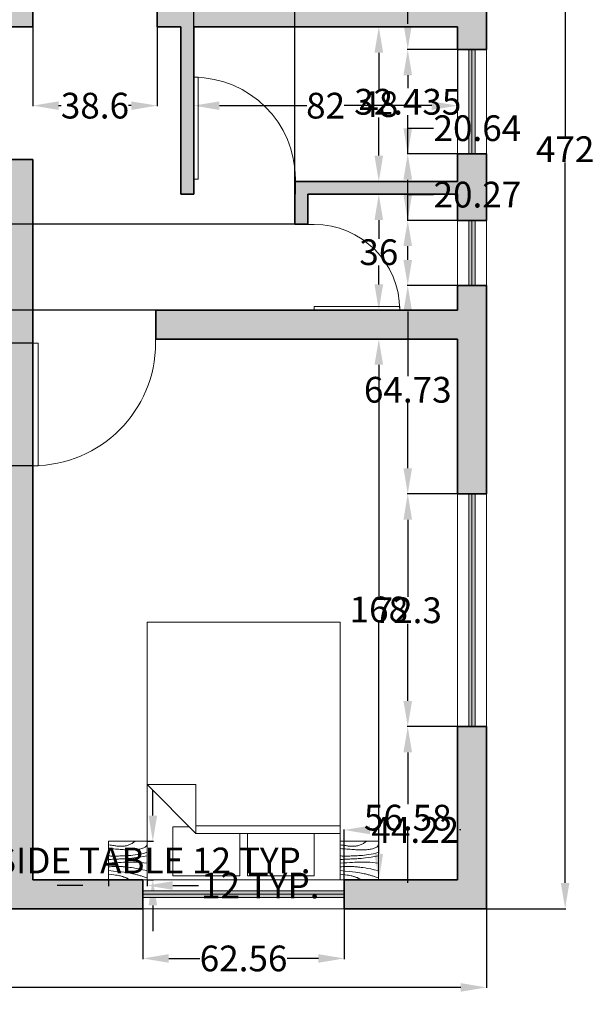
# Model space of a CAD drawing. Units: inches. Extents: x -52 to 678, y 23 to 685.
# Tile 10 of 11: x 431 to 609, y 23 to 329. Entities that reach past the tile are written whole.
import ezdxf

# ---------------------------------------------------------------- set-up
doc = ezdxf.new("R2010")
doc.units = ezdxf.units.IN
doc.header["$MEASUREMENT"] = 0
for name, color, linetype, lineweight in [('A-ANNO-DIMS', 2, 'Continuous', 18), ('A-DOOR', 3, 'Continuous', 18), ('A-FURN', 8, 'Continuous', 18), ('A-GLAZ', 4, 'Continuous', 18), ('A-WALL', 7, 'Continuous', 35)]:
    doc.layers.add(name, color=color, linetype=linetype, lineweight=lineweight)
doc.layers.add('A-GLAZ-PATT', color=18, linetype='Continuous', lineweight=13, true_color=0x000000)
doc.layers.add('A-WALL-PATT', color=18, linetype='Continuous', lineweight=13, true_color=0x000000)
doc.styles.get("Standard").update_dxf_attribs({"font": 'arial.ttf'})
doc.dimstyles.get("Standard").update_dxf_attribs({"dimtxt": 8, "dimasz": 8, "dimexe": 0.18, "dimexo": 0.0625, "dimgap": 0.09, "dimtad": 0, "dimtih": 1, "dimtoh": 1, "dimdec": 0, "dimzin": 0, "dimdsep": 46, "dimlunit": 3, "dimtxsty": 'Standard', "dimcen": 0.09, "dimadec": 0, "dimazin": 0, "dimtfac": 1, "dimtdec": 0, "dimtofl": 0, "dimtmove": 0, "dimatfit": 3, "dimfxl": 1, "dimtolj": 1, "dimtzin": 0, "dimarcsym": 0})

# ---------------------------------------------------------------- blocks, each defined once
blk = doc.blocks.new('Bed - Queen')
for p, q in [((0, -80.00003), (0, 0)), ((0, 0), (59.99999, 0)), ((59.99999, 0), (59.99999, -80.00003)), ((7.99999, -1.2), (28.79998, -1.2)), ((7.99999, -14.4), (7.99999, -1.2)), ((28.79998, -1.2), (28.79998, -14.4)), ((31.19999, -1.2), (51.99999, -1.2)), ((31.19999, -14.4), (31.19999, -1.2)), ((51.99999, -1.2), (51.99999, -16.4)), ((0, -14.4), (44.8, -14.4)), ((59.99999, -29.6), (44.8, -14.4)), ((44.8, -14.4), (44.8, -29.6)), ((44.8, -16.8), (0, -16.8)), ((51.99999, -16.4), (46.79936, -16.4)), ((44.8, -29.6), (59.99999, -29.6)), ((59.99999, -80.00003), (0, -80.00003))]:
    blk.add_line(p, q)
blk = doc.blocks.new('Table - Square Woodgrain 42 x 42 in.')
blk.add_line((0, -42), (42, -42))
for points in [[(0, -4), (1.704, -4.2172), (3.2358, -4.4188), (4.615, -4.604), (5.8615, -4.7721), (6.9951, -4.9224), (8.0357, -5.0541), (9.0031, -5.1667), (9.9171, -5.2594), (10.7951, -5.3316), (11.6445, -5.3836), (12.4702, -5.4157), (13.277, -5.4283), (14.0698, -5.4217), (14.8535, -5.3964), (15.6331, -5.3526), (16.4133, -5.2908), (17.1986, -5.2103), (17.9913, -5.1062), (18.793, -4.9727), (19.6056, -4.8038), (20.4307, -4.5937), (21.2701, -4.3365), (22.1256, -4.0262), (22.9989, -3.6571), (23.888, -3.2272), (24.7756, -2.7516), (25.6408, -2.2491), (26.4624, -1.7387), (27.2195, -1.2395), (27.891, -0.7703), (28.456, -0.3501), (28.8934, 0.002)], [(0, -42), (0, 0), (42, 0), (42, -42)], [(0, -8), (1.8203, -8.1001), (3.6741, -8.2149), (5.5411, -8.3408), (7.4011, -8.4741), (9.2339, -8.6112), (11.0193, -8.7484), (12.7371, -8.8821), (14.3671, -9.0086), (15.8954, -9.1246), (17.3337, -9.2278), (18.6997, -9.3159), (20.0116, -9.387), (21.2871, -9.4389), (22.5442, -9.4696), (23.8008, -9.477), (25.0749, -9.459), (26.3791, -9.4137), (27.7049, -9.3403), (29.0383, -9.2382), (30.3655, -9.1068), (31.6728, -8.9455), (32.9461, -8.7535), (34.1717, -8.5304), (35.3358, -8.2756), (36.4268, -7.9863), (37.443, -7.6521), (38.3849, -7.2603), (39.253, -6.7986), (40.048, -6.2542), (40.7705, -5.6147), (41.421, -4.8674), (42, -4)], [(42, -12), (39.1784, -12.8621), (36.4519, -13.5654), (33.8246, -14.1294), (31.3004, -14.5731), (28.8832, -14.9161), (26.577, -15.1775), (24.3858, -15.3768), (22.3136, -15.5332), (20.3622, -15.6632), (18.5254, -15.7718), (16.7947, -15.8612), (15.1618, -15.9338), (13.6183, -15.9916), (12.1558, -16.0369), (10.7659, -16.0718), (9.4403, -16.0987), (8.1703, -16.1191), (6.9461, -16.1325), (5.7577, -16.1377), (4.595, -16.1335), (3.4479, -16.1188), (2.3064, -16.0924), (1.1604, -16.0532), (0, -16)], [(42, -16), (37.6529, -16.7365), (33.8802, -17.329), (30.6179, -17.7961), (27.8015, -18.1561), (25.3668, -18.4275), (23.2497, -18.6288), (21.3859, -18.7785), (19.7111, -18.8949), (18.1693, -18.9939), (16.7375, -19.0795), (15.401, -19.1534), (14.1449, -19.217), (12.9544, -19.2717), (11.8148, -19.3191), (10.7113, -19.3606), (9.6291, -19.3976), (8.5534, -19.4323), (7.47, -19.4689), (6.3643, -19.5122), (5.222, -19.5672), (4.0288, -19.6386), (2.7703, -19.7313), (1.4321, -19.8501), (0, -20)], [(0, -24), (3.9243, -23.6805), (7.4766, -23.4138), (10.6891, -23.1954), (13.5943, -23.0205), (16.2247, -22.8847), (18.6125, -22.7832), (20.7903, -22.7116), (22.7903, -22.6651), (24.6563, -22.642), (26.4764, -22.6507), (28.35, -22.7024), (30.3766, -22.8084), (32.6555, -22.98), (35.2861, -23.2283), (38.3678, -23.5645), (42, -24)], [(42, -32), (37.392, -31.017), (33.4585, -30.2231), (30.1291, -29.5949), (27.3334, -29.109), (25.0009, -28.742), (23.0612, -28.4707), (21.4439, -28.2716), (20.0786, -28.1215), (18.8998, -28.0002), (17.8609, -27.9014), (16.9206, -27.8219), (16.0371, -27.7588), (15.1691, -27.709), (14.2748, -27.6693), (13.3128, -27.6368), (12.2415, -27.6083), (11.0295, -27.5824), (9.6867, -27.5643), (8.233, -27.5608), (6.6884, -27.5787), (5.0728, -27.6248), (3.4062, -27.7058), (1.7086, -27.8286), (0, -28)], [(0, -32), (5.4026, -32.5358), (9.9494, -33.019), (13.7424, -33.4553), (16.8834, -33.8505), (19.4743, -34.2106), (21.6171, -34.5413), (23.4136, -34.8486), (24.9657, -35.1382), (26.3614, -35.4156), (27.6332, -35.6841), (28.7995, -35.9467), (29.8788, -36.2064), (30.8897, -36.4661), (31.8507, -36.7288), (32.7802, -36.9973), (33.6968, -37.2747), (34.6175, -37.5635), (35.5531, -37.8651), (36.5128, -38.1805), (37.506, -38.5108), (38.5421, -38.8568), (39.6302, -39.2197), (40.7797, -39.6004), (42, -40)], [(0, -36), (3.0098, -36.2857), (5.5354, -36.5643), (7.6368, -36.8359), (9.374, -37.1009), (10.807, -37.3597), (11.9957, -37.6126), (13.0002, -37.8599), (13.8804, -38.102), (14.6874, -38.3393), (15.4365, -38.5729), (16.1338, -38.8041), (16.7858, -39.0341), (17.3987, -39.264), (17.9787, -39.4952), (18.5322, -39.7288), (19.0655, -39.9662), (19.5832, -40.2081), (20.0842, -40.4544), (20.5657, -40.7046), (21.0249, -40.9581), (21.459, -41.2144), (21.8653, -41.4731), (22.2409, -41.7335), (22.5831, -41.9951)]]:
    blk.add_lwpolyline(points)
blk = doc.blocks.new('*U15')
for p, q in [((0, 0), (0, -6)), ((-40, 0), (-40, -6))]:
    blk.add_line(p, q)
blk.add_lwpolyline([(0, 0), (0, 40), (-1.75, 40), (-1.75, 0)], close=True)
blk.add_arc((0, 0), 40, 90, 180)
blk = doc.blocks.new('*U14')
for p, q in [((0, 0), (0, -6)), ((40, 0), (40, -6))]:
    blk.add_line(p, q)
blk.add_lwpolyline([(0, 0), (0, 40), (1.75, 40), (1.75, 0)], close=True)
blk.add_arc((0, 0), 40, 0, 90)
blk = doc.blocks.new('*D17')
at = {"layer": 'A-ANNO-DIMS', "color": 0, "lineweight": -2, "transparency": 16777216}
for p, q in [((471.9, 82.07), (471.9, 90.07)), ((470.17, 74.07), (472.08, 74.07)), ((470.17, 62.13), (472.08, 62.13)), ((471.9, 54.13), (471.9, 46.13))]:
    blk.add_line(p, q, dxfattribs=at)
at = {"layer": 'A-ANNO-DIMS', "color": 0, "transparency": 16777216}
for points in [[(470.56, 82.07), (473.23, 82.07), (471.9, 74.07)], [(470.56, 54.13), (473.23, 54.13), (471.9, 62.13)]]:
    blk.add_solid(points, dxfattribs=at)
at = {"layer": 'Defpoints', "color": 0, "transparency": 16777216}
for p in [(470.1, 74.07), (471.9, 74.07), (470.1, 62.13)]:
    blk.add_point(p, dxfattribs=at)
at = {"layer": 'A-ANNO-DIMS', "color": 0, "transparency": 16777216, "insert": (471.9, 68.1), "char_height": 8, "attachment_point": 5}
blk.add_mtext('\\A1;SIDE TABLE 12 TYP.', dxfattribs=at)
blk = doc.blocks.new('*D18')
at = {"layer": 'A-ANNO-DIMS', "color": 0, "lineweight": -2, "transparency": 16777216}
for p, q in [((458.16, 62.06), (458.16, 60.15)), ((470.1, 62.06), (470.1, 60.15)), ((450.16, 60.33), (442.16, 60.33)), ((478.1, 60.33), (486.1, 60.33))]:
    blk.add_line(p, q, dxfattribs=at)
at = {"layer": 'A-ANNO-DIMS', "color": 0, "transparency": 16777216}
for points in [[(450.16, 61.67), (450.16, 59), (458.16, 60.33)], [(478.1, 61.67), (478.1, 59), (470.1, 60.33)]]:
    blk.add_solid(points, dxfattribs=at)
at = {"layer": 'Defpoints', "color": 0, "transparency": 16777216}
for p in [(458.16, 62.13), (470.1, 62.13), (470.1, 60.33)]:
    blk.add_point(p, dxfattribs=at)
at = {"layer": 'A-ANNO-DIMS', "color": 0, "transparency": 16777216, "insert": (505.29, 60.33), "char_height": 8, "attachment_point": 5}
blk.add_mtext('\\A1;12 TYP.', dxfattribs=at)
blk = doc.blocks.new('*D39')
at = {"layer": 'A-ANNO-DIMS', "color": 0, "lineweight": -2, "transparency": 16777216}
for p, q in [((91.61, 327.06), (91.61, 28.49)), ((575.61, 53.06), (575.61, 28.49)), ((99.61, 28.67), (324.53, 28.67)), ((567.61, 28.67), (342.68, 28.67))]:
    blk.add_line(p, q, dxfattribs=at)
at = {"layer": 'A-ANNO-DIMS', "color": 0, "transparency": 16777216}
for points in [[(99.61, 30), (99.61, 27.33), (91.61, 28.67)], [(567.61, 30), (567.61, 27.33), (575.61, 28.67)]]:
    blk.add_solid(points, dxfattribs=at)
at = {"layer": 'Defpoints', "color": 0, "transparency": 16777216}
for p in [(91.61, 327.13), (575.61, 53.13), (575.61, 28.67)]:
    blk.add_point(p, dxfattribs=at)
at = {"layer": 'A-ANNO-DIMS', "color": 0, "transparency": 16777216, "insert": (333.61, 28.67), "char_height": 8, "attachment_point": 5}
blk.add_mtext('\\A1;484', dxfattribs=at)
blk = doc.blocks.new('*D40')
at = {"layer": 'A-ANNO-DIMS', "color": 0, "lineweight": -2, "transparency": 16777216}
for p, q in [((358.67, 525.13), (600.25, 525.13)), ((600.07, 517.13), (600.07, 293.23)), ((600.07, 61.13), (600.07, 285.02)), ((575.67, 53.13), (600.25, 53.13))]:
    blk.add_line(p, q, dxfattribs=at)
at = {"layer": 'A-ANNO-DIMS', "color": 0, "transparency": 16777216}
for points in [[(598.73, 517.13), (601.4, 517.13), (600.07, 525.13)], [(598.73, 61.13), (601.4, 61.13), (600.07, 53.13)]]:
    blk.add_solid(points, dxfattribs=at)
at = {"layer": 'Defpoints', "color": 0, "transparency": 16777216}
for p in [(358.61, 525.13), (600.07, 525.13), (575.61, 53.13)]:
    blk.add_point(p, dxfattribs=at)
at = {"layer": 'A-ANNO-DIMS', "color": 0, "transparency": 16777216, "insert": (600.07, 289.13), "char_height": 8, "attachment_point": 5}
blk.add_mtext('\\A1;472', dxfattribs=at)
blk = doc.blocks.new('*D51')
at = {"layer": 'A-ANNO-DIMS', "color": 0, "lineweight": -2, "transparency": 16777216}
for p, q in [((566.54, 230.13), (541.97, 230.13)), ((542.15, 222.13), (542.15, 150.3)), ((542.15, 70.13), (542.15, 141.95)), ((566.54, 62.13), (541.97, 62.13))]:
    blk.add_line(p, q, dxfattribs=at)
at = {"layer": 'A-ANNO-DIMS', "color": 0, "transparency": 16777216}
for points in [[(540.81, 222.13), (543.48, 222.13), (542.15, 230.13)], [(540.81, 70.13), (543.48, 70.13), (542.15, 62.13)]]:
    blk.add_solid(points, dxfattribs=at)
at = {"layer": 'Defpoints', "color": 0, "transparency": 16777216}
for p in [(542.15, 230.13), (566.61, 230.13), (566.61, 62.13)]:
    blk.add_point(p, dxfattribs=at)
at = {"layer": 'A-ANNO-DIMS', "color": 0, "transparency": 16777216, "insert": (542.15, 146.13), "char_height": 8, "attachment_point": 5}
blk.add_mtext('\\A1;168', dxfattribs=at)
blk = doc.blocks.new('*D52')
at = {"layer": 'A-ANNO-DIMS', "color": 0, "lineweight": -2, "transparency": 16777216}
for p, q in [((566.54, 275.13), (541.97, 275.13)), ((542.15, 267.13), (542.15, 261.3)), ((542.15, 247.13), (542.15, 252.95)), ((566.54, 239.13), (541.97, 239.13))]:
    blk.add_line(p, q, dxfattribs=at)
at = {"layer": 'A-ANNO-DIMS', "color": 0, "transparency": 16777216}
for points in [[(540.81, 267.13), (543.48, 267.13), (542.15, 275.13)], [(540.81, 247.13), (543.48, 247.13), (542.15, 239.13)]]:
    blk.add_solid(points, dxfattribs=at)
at = {"layer": 'Defpoints', "color": 0, "transparency": 16777216}
for p in [(542.15, 275.13), (566.61, 275.13), (566.61, 239.13)]:
    blk.add_point(p, dxfattribs=at)
at = {"layer": 'A-ANNO-DIMS', "color": 0, "transparency": 16777216, "insert": (542.15, 257.13), "char_height": 8, "attachment_point": 5}
blk.add_mtext('\\A1;36', dxfattribs=at)
blk = doc.blocks.new('*D55')
at = {"layer": 'A-ANNO-DIMS', "color": 0, "lineweight": -2, "transparency": 16777216}
for p, q in [((484.61, 327.06), (484.61, 302.49)), ((566.61, 327.06), (566.61, 302.49)), ((492.61, 302.67), (519.82, 302.67)), ((558.61, 302.67), (531.39, 302.67))]:
    blk.add_line(p, q, dxfattribs=at)
at = {"layer": 'A-ANNO-DIMS', "color": 0, "transparency": 16777216}
for points in [[(492.61, 304), (492.61, 301.33), (484.61, 302.67)], [(558.61, 304), (558.61, 301.33), (566.61, 302.67)]]:
    blk.add_solid(points, dxfattribs=at)
at = {"layer": 'Defpoints', "color": 0, "transparency": 16777216}
for p in [(484.61, 327.13), (566.61, 327.13), (484.61, 302.67)]:
    blk.add_point(p, dxfattribs=at)
at = {"layer": 'A-ANNO-DIMS', "color": 0, "transparency": 16777216, "insert": (525.61, 302.67), "char_height": 8, "attachment_point": 5}
blk.add_mtext('\\A1;82', dxfattribs=at)
blk = doc.blocks.new('*D56')
at = {"layer": 'A-ANNO-DIMS', "color": 0, "lineweight": -2, "transparency": 16777216}
for p, q in [((566.54, 327.13), (541.97, 327.13)), ((542.15, 319.13), (542.15, 307.3)), ((542.15, 287.13), (542.15, 298.95)), ((566.54, 279.13), (541.97, 279.13))]:
    blk.add_line(p, q, dxfattribs=at)
at = {"layer": 'A-ANNO-DIMS', "color": 0, "transparency": 16777216}
for points in [[(540.81, 319.13), (543.48, 319.13), (542.15, 327.13)], [(540.81, 287.13), (543.48, 287.13), (542.15, 279.13)]]:
    blk.add_solid(points, dxfattribs=at)
at = {"layer": 'Defpoints', "color": 0, "transparency": 16777216}
for p in [(542.15, 327.13), (566.61, 327.13), (566.61, 279.13)]:
    blk.add_point(p, dxfattribs=at)
at = {"layer": 'A-ANNO-DIMS', "color": 0, "transparency": 16777216, "insert": (542.15, 303.13), "char_height": 8, "attachment_point": 5}
blk.add_mtext('\\A1;48', dxfattribs=at)
blk = doc.blocks.new('*D69')
at = {"layer": 'A-ANNO-DIMS', "color": 0, "lineweight": -2, "transparency": 16777216}
for p, q in [((434.61, 327.06), (434.61, 302.49)), ((473.2, 327.06), (473.2, 302.49)), ((442.61, 302.67), (443.43, 302.67)), ((465.2, 302.67), (464.38, 302.67))]:
    blk.add_line(p, q, dxfattribs=at)
at = {"layer": 'A-ANNO-DIMS', "color": 0, "transparency": 16777216}
for points in [[(442.61, 304), (442.61, 301.33), (434.61, 302.67)], [(465.2, 304), (465.2, 301.33), (473.2, 302.67)]]:
    blk.add_solid(points, dxfattribs=at)
at = {"layer": 'Defpoints', "color": 0, "transparency": 16777216}
for p in [(434.61, 327.13), (473.2, 327.13), (434.61, 302.67)]:
    blk.add_point(p, dxfattribs=at)
at = {"layer": 'A-ANNO-DIMS', "color": 0, "transparency": 16777216, "insert": (453.9, 302.67), "char_height": 8, "attachment_point": 5}
blk.add_mtext('\\A1;38.6', dxfattribs=at)
blk = doc.blocks.new('*D88')
at = {"layer": 'A-ANNO-DIMS', "color": 0, "lineweight": -2, "transparency": 16777216}
for p, q in [((575.54, 109.71), (550.97, 109.71)), ((551.15, 101.71), (551.15, 85.59)), ((551.15, 61.13), (551.15, 77.24)), ((575.54, 53.13), (550.97, 53.13))]:
    blk.add_line(p, q, dxfattribs=at)
at = {"layer": 'A-ANNO-DIMS', "color": 0, "transparency": 16777216}
for points in [[(549.81, 101.71), (552.48, 101.71), (551.15, 109.71)], [(549.81, 61.13), (552.48, 61.13), (551.15, 53.13)]]:
    blk.add_solid(points, dxfattribs=at)
at = {"layer": 'Defpoints', "color": 0, "transparency": 16777216}
for p in [(551.15, 109.71), (575.61, 109.71), (575.61, 53.13)]:
    blk.add_point(p, dxfattribs=at)
at = {"layer": 'A-ANNO-DIMS', "color": 0, "transparency": 16777216, "insert": (551.15, 81.42), "char_height": 8, "attachment_point": 5}
blk.add_mtext('\\A1;56.58', dxfattribs=at)
blk = doc.blocks.new('*D89')
at = {"layer": 'A-ANNO-DIMS', "color": 0, "lineweight": -2, "transparency": 16777216}
for p, q in [((575.54, 182.01), (550.97, 182.01)), ((551.15, 174.01), (551.15, 150.04)), ((551.15, 117.71), (551.15, 141.68)), ((575.54, 109.71), (550.97, 109.71))]:
    blk.add_line(p, q, dxfattribs=at)
at = {"layer": 'A-ANNO-DIMS', "color": 0, "transparency": 16777216}
for points in [[(549.81, 174.01), (552.48, 174.01), (551.15, 182.01)], [(549.81, 117.71), (552.48, 117.71), (551.15, 109.71)]]:
    blk.add_solid(points, dxfattribs=at)
at = {"layer": 'Defpoints', "color": 0, "transparency": 16777216}
for p in [(551.15, 182.01), (575.61, 182.01), (575.61, 109.71)]:
    blk.add_point(p, dxfattribs=at)
at = {"layer": 'A-ANNO-DIMS', "color": 0, "transparency": 16777216, "insert": (551.15, 145.86), "char_height": 8, "attachment_point": 5}
blk.add_mtext('\\A1;72.3', dxfattribs=at)
blk = doc.blocks.new('*D90')
at = {"layer": 'A-ANNO-DIMS', "color": 0, "lineweight": -2, "transparency": 16777216}
for p, q in [((575.54, 246.74), (550.97, 246.74)), ((551.15, 238.74), (551.15, 218.56)), ((551.15, 190.01), (551.15, 210.2)), ((575.54, 182.01), (550.97, 182.01))]:
    blk.add_line(p, q, dxfattribs=at)
at = {"layer": 'A-ANNO-DIMS', "color": 0, "transparency": 16777216}
for points in [[(549.81, 238.74), (552.48, 238.74), (551.15, 246.74)], [(549.81, 190.01), (552.48, 190.01), (551.15, 182.01)]]:
    blk.add_solid(points, dxfattribs=at)
at = {"layer": 'Defpoints', "color": 0, "transparency": 16777216}
for p in [(551.15, 246.74), (575.61, 246.74), (575.61, 182.01)]:
    blk.add_point(p, dxfattribs=at)
at = {"layer": 'A-ANNO-DIMS', "color": 0, "transparency": 16777216, "insert": (551.15, 214.38), "char_height": 8, "attachment_point": 5}
blk.add_mtext('\\A1;64.73', dxfattribs=at)
blk = doc.blocks.new('*D91')
at = {"layer": 'A-ANNO-DIMS', "color": 0, "lineweight": -2, "transparency": 16777216}
for p, q in [((551.15, 267.02), (551.15, 275.02)), ((551.15, 275.02), (559.15, 275.02)), ((575.54, 267.02), (550.97, 267.02)), ((551.15, 254.74), (551.15, 259.02)), ((575.54, 246.74), (550.97, 246.74))]:
    blk.add_line(p, q, dxfattribs=at)
at = {"layer": 'A-ANNO-DIMS', "color": 0, "transparency": 16777216}
for points in [[(549.81, 259.02), (552.48, 259.02), (551.15, 267.02)], [(549.81, 254.74), (552.48, 254.74), (551.15, 246.74)]]:
    blk.add_solid(points, dxfattribs=at)
at = {"layer": 'Defpoints', "color": 0, "transparency": 16777216}
for p in [(551.15, 267.02), (575.61, 267.02), (575.61, 246.74)]:
    blk.add_point(p, dxfattribs=at)
at = {"layer": 'A-ANNO-DIMS', "color": 0, "transparency": 16777216, "insert": (572.8, 275.02), "char_height": 8, "attachment_point": 5}
blk.add_mtext('\\A1;20.27', dxfattribs=at)
blk = doc.blocks.new('*D92')
at = {"layer": 'A-ANNO-DIMS', "color": 0, "lineweight": -2, "transparency": 16777216}
for p, q in [((551.15, 287.66), (551.15, 295.66)), ((551.15, 295.66), (559.15, 295.66)), ((575.54, 287.66), (550.97, 287.66)), ((551.15, 275.02), (551.15, 279.66)), ((575.54, 267.02), (550.97, 267.02))]:
    blk.add_line(p, q, dxfattribs=at)
at = {"layer": 'A-ANNO-DIMS', "color": 0, "transparency": 16777216}
for points in [[(549.81, 279.66), (552.48, 279.66), (551.15, 287.66)], [(549.81, 275.02), (552.48, 275.02), (551.15, 267.02)]]:
    blk.add_solid(points, dxfattribs=at)
at = {"layer": 'Defpoints', "color": 0, "transparency": 16777216}
for p in [(551.15, 287.66), (575.61, 287.66), (575.61, 267.02)]:
    blk.add_point(p, dxfattribs=at)
at = {"layer": 'A-ANNO-DIMS', "color": 0, "transparency": 16777216, "insert": (572.79, 295.66), "char_height": 8, "attachment_point": 5}
blk.add_mtext('\\A1;20.64', dxfattribs=at)
blk = doc.blocks.new('*D93')
at = {"layer": 'A-ANNO-DIMS', "color": 0, "lineweight": -2, "transparency": 16777216}
for p, q in [((575.54, 320.09), (550.97, 320.09)), ((551.15, 312.09), (551.15, 308.05)), ((551.15, 295.66), (551.15, 299.7)), ((575.54, 287.66), (550.97, 287.66))]:
    blk.add_line(p, q, dxfattribs=at)
at = {"layer": 'A-ANNO-DIMS', "color": 0, "transparency": 16777216}
for points in [[(549.81, 312.09), (552.48, 312.09), (551.15, 320.09)], [(549.81, 295.66), (552.48, 295.66), (551.15, 287.66)]]:
    blk.add_solid(points, dxfattribs=at)
at = {"layer": 'Defpoints', "color": 0, "transparency": 16777216}
for p in [(551.15, 320.09), (575.61, 320.09), (575.61, 287.66)]:
    blk.add_point(p, dxfattribs=at)
at = {"layer": 'A-ANNO-DIMS', "color": 0, "transparency": 16777216, "insert": (551.15, 303.87), "char_height": 8, "attachment_point": 5}
blk.add_mtext('\\A1;32.435', dxfattribs=at)
blk = doc.blocks.new('*D94')
at = {"layer": 'A-ANNO-DIMS', "color": 0, "lineweight": -2, "transparency": 16777216}
for p, q in [((575.54, 366.32), (550.97, 366.32)), ((551.15, 358.32), (551.15, 347.38)), ((551.15, 328.09), (551.15, 339.03)), ((575.54, 320.09), (550.97, 320.09))]:
    blk.add_line(p, q, dxfattribs=at)
at = {"layer": 'A-ANNO-DIMS', "color": 0, "transparency": 16777216}
for points in [[(549.81, 358.32), (552.48, 358.32), (551.15, 366.32)], [(549.81, 328.09), (552.48, 328.09), (551.15, 320.09)]]:
    blk.add_solid(points, dxfattribs=at)
at = {"layer": 'Defpoints', "color": 0, "transparency": 16777216}
for p in [(551.15, 366.32), (575.61, 366.32), (575.61, 320.09)]:
    blk.add_point(p, dxfattribs=at)
at = {"layer": 'A-ANNO-DIMS', "color": 0, "transparency": 16777216, "insert": (551.15, 343.21), "char_height": 8, "attachment_point": 5}
blk.add_mtext('\\A1;46.23', dxfattribs=at)
blk = doc.blocks.new('*D96')
at = {"layer": 'A-ANNO-DIMS', "color": 0, "lineweight": -2, "transparency": 16777216}
for p, q in [((468.83, 62.06), (468.83, 37.49)), ((531.38, 62.06), (531.38, 37.49)), ((476.83, 37.67), (486.5, 37.67)), ((523.38, 37.67), (513.71, 37.67))]:
    blk.add_line(p, q, dxfattribs=at)
at = {"layer": 'A-ANNO-DIMS', "color": 0, "transparency": 16777216}
for points in [[(476.83, 39), (476.83, 36.33), (468.83, 37.67)], [(523.38, 39), (523.38, 36.33), (531.38, 37.67)]]:
    blk.add_solid(points, dxfattribs=at)
at = {"layer": 'Defpoints', "color": 0, "transparency": 16777216}
for p in [(468.83, 62.13), (531.38, 62.13), (468.83, 37.67)]:
    blk.add_point(p, dxfattribs=at)
at = {"layer": 'A-ANNO-DIMS', "color": 0, "transparency": 16777216, "insert": (500.1, 37.67), "char_height": 8, "attachment_point": 5}
blk.add_mtext('\\A1;62.56', dxfattribs=at)
blk = doc.blocks.new('*D97')
at = {"layer": 'A-ANNO-DIMS', "color": 0, "lineweight": -2, "transparency": 16777216}
for p, q in [((531.38, 53.19), (531.38, 77.77)), ((539.38, 77.59), (539.79, 77.59)), ((567.61, 77.59), (567.2, 77.59)), ((575.61, 53.19), (575.61, 77.77))]:
    blk.add_line(p, q, dxfattribs=at)
at = {"layer": 'A-ANNO-DIMS', "color": 0, "transparency": 16777216}
for points in [[(539.38, 78.92), (539.38, 76.25), (531.38, 77.59)], [(567.61, 78.92), (567.61, 76.25), (575.61, 77.59)]]:
    blk.add_solid(points, dxfattribs=at)
at = {"layer": 'Defpoints', "color": 0, "transparency": 16777216}
for p in [(575.61, 77.59), (531.38, 53.13), (575.61, 53.13)]:
    blk.add_point(p, dxfattribs=at)
at = {"layer": 'A-ANNO-DIMS', "color": 0, "transparency": 16777216, "insert": (553.49, 77.59), "char_height": 8, "attachment_point": 5}
blk.add_mtext('\\A1;44.22', dxfattribs=at)
blk = doc.blocks.new('*D98')
at = {"layer": 'A-ANNO-DIMS', "color": 0, "lineweight": -2, "transparency": 16777216}
for p, q in [((434.54, 228.91), (409.97, 228.91)), ((410.15, 220.91), (410.15, 214.02)), ((410.15, 198.77), (410.15, 205.66)), ((434.54, 190.77), (409.97, 190.77))]:
    blk.add_line(p, q, dxfattribs=at)
at = {"layer": 'A-ANNO-DIMS', "color": 0, "transparency": 16777216}
for points in [[(408.81, 220.91), (411.48, 220.91), (410.15, 228.91)], [(408.81, 198.77), (411.48, 198.77), (410.15, 190.77)]]:
    blk.add_solid(points, dxfattribs=at)
at = {"layer": 'Defpoints', "color": 0, "transparency": 16777216}
for p in [(410.15, 228.91), (434.61, 228.91), (434.61, 190.77)]:
    blk.add_point(p, dxfattribs=at)
at = {"layer": 'A-ANNO-DIMS', "color": 0, "transparency": 16777216, "insert": (410.15, 209.84), "char_height": 8, "attachment_point": 5}
blk.add_mtext('\\A1;38.13', dxfattribs=at)
blk = doc.blocks.new('*D99')
at = {"layer": 'A-ANNO-DIMS', "color": 0, "lineweight": -2, "transparency": 16777216}
for p, q in [((484.61, 275.19), (484.61, 549.77)), ((492.61, 549.59), (508.05, 549.59)), ((516.05, 279.19), (516.05, 549.77)), ((516.05, 549.59), (524.05, 549.59))]:
    blk.add_line(p, q, dxfattribs=at)
at = {"layer": 'A-ANNO-DIMS', "color": 0, "transparency": 16777216}
for points in [[(492.61, 550.92), (492.61, 548.25), (484.61, 549.59)], [(508.05, 550.92), (508.05, 548.25), (516.05, 549.59)]]:
    blk.add_solid(points, dxfattribs=at)
at = {"layer": 'Defpoints', "color": 0, "transparency": 16777216}
for p in [(516.05, 549.59), (516.05, 279.13), (484.61, 275.13)]:
    blk.add_point(p, dxfattribs=at)
at = {"layer": 'A-ANNO-DIMS', "color": 0, "transparency": 16777216, "insert": (540.74, 549.59), "char_height": 8, "attachment_point": 5}
blk.add_mtext('\\A1;31.446', dxfattribs=at)
blk = doc.blocks.new('*D100')
at = {"layer": 'A-ANNO-DIMS', "color": 0, "lineweight": -2, "transparency": 16777216}
for p, q in [((519.99, 265.81), (66.97, 265.81)), ((67.15, 257.81), (67.15, 256.65)), ((67.15, 247.13), (67.15, 248.3)), ((521.98, 239.13), (66.97, 239.13))]:
    blk.add_line(p, q, dxfattribs=at)
at = {"layer": 'A-ANNO-DIMS', "color": 0, "transparency": 16777216}
for points in [[(65.81, 257.81), (68.48, 257.81), (67.15, 265.81)], [(65.81, 247.13), (68.48, 247.13), (67.15, 239.13)]]:
    blk.add_solid(points, dxfattribs=at)
at = {"layer": 'Defpoints', "color": 0, "transparency": 16777216}
for p in [(520.05, 265.81), (67.15, 239.13), (522.04, 239.13)]:
    blk.add_point(p, dxfattribs=at)
at = {"layer": 'A-ANNO-DIMS', "color": 0, "transparency": 16777216, "insert": (67.15, 252.47), "char_height": 8, "attachment_point": 5}
blk.add_mtext('\\A1;26.69', dxfattribs=at)

msp = doc.modelspace()

# ---------------------------------------------------------------- hatches: boundary and pattern name
at = {"layer": 'A-GLAZ-PATT'}
h = msp.add_hatch(color=256, dxfattribs=at)
h.dxf.hatch_style = 1
h.paths.add_polyline_path([(570.1053, 287.6563), (571.1053, 287.6563), (571.1053, 320.0909), (570.1053, 320.0909)])
h = msp.add_hatch(color=256, dxfattribs=at)
h.dxf.hatch_style = 1
h.paths.add_polyline_path([(571.1053, 287.6563), (572.1053, 287.6563), (572.1053, 320.0909), (571.1053, 320.0909)])
h = msp.add_hatch(color=256, dxfattribs=at)
h.dxf.hatch_style = 1
h.paths.add_polyline_path([(571.1053, 267.0161), (570.1053, 267.0161), (570.1053, 246.7445), (571.1053, 246.7445)])
h = msp.add_hatch(color=256, dxfattribs=at)
h.dxf.hatch_style = 1
h.paths.add_polyline_path([(571.1053, 246.7445), (572.1053, 246.7445), (572.1053, 267.0161), (571.1053, 267.0161)])
h = msp.add_hatch(color=256, dxfattribs=at)
h.dxf.hatch_style = 1
h.paths.add_polyline_path([(570.1053, 109.7091), (571.1053, 109.7091), (571.1053, 182.0114), (570.1053, 182.0114)])
h = msp.add_hatch(color=256, dxfattribs=at)
h.dxf.hatch_style = 1
h.paths.add_polyline_path([(571.1053, 109.7091), (572.1053, 109.7091), (572.1053, 182.0114), (571.1053, 182.0114)])
h = msp.add_hatch(color=256, dxfattribs=at)
h.dxf.hatch_style = 1
h.paths.add_polyline_path([(531.3824, 57.6267), (531.3824, 58.6267), (468.8253, 58.6267), (468.8253, 57.6267)])
h = msp.add_hatch(color=256, dxfattribs=at)
h.dxf.hatch_style = 1
h.paths.add_polyline_path([(468.8253, 57.6267), (468.8253, 56.6267), (531.3824, 56.6267), (531.3824, 57.6267)])
at = {"layer": 'A-WALL-PATT'}
h = msp.add_hatch(color=256, dxfattribs=at)
h.dxf.hatch_style = 1
h.paths.add_polyline_path([(349.6053, 340.107), (349.6053, 327.1267), (410.6053, 327.1267), (434.6053, 327.1267), (434.6053, 336.1267), (410.6053, 336.1267), (410.6053, 340.107), (410.6053, 363.4905), (406.6053, 363.4905), (406.6053, 340.107), (406.6053, 336.1267), (358.6053, 336.1267), (358.6053, 340.107), (358.6053, 392.1267), (382.6053, 392.1267), (382.6053, 396.1267), (358.6053, 396.1267), (358.6053, 468.1267), (372.5751, 468.1267), (372.5751, 477.1267), (358.6053, 477.1267), (358.6053, 525.1267), (341.0247, 525.1267), (341.0247, 516.1267), (349.6053, 516.1267)])
h = msp.add_hatch(color=256, dxfattribs=at)
h.dxf.hatch_style = 1
h.paths.add_polyline_path([(575.6053, 366.3195), (566.6053, 366.3195), (566.6053, 336.1267), (473.2028, 336.1267), (473.2028, 327.1267), (480.6053, 327.1267), (480.6053, 275.1267), (484.6053, 275.1267), (484.6053, 327.1267), (566.6053, 327.1267), (566.6053, 320.0909), (575.6053, 320.0909)])
h = msp.add_hatch(color=256, dxfattribs=at)
h.dxf.hatch_style = 1
h.paths.add_polyline_path([(566.6053, 279.1267), (516.0511, 279.1267), (516.0511, 275.1267), (516.0511, 265.8145), (520.0511, 265.8145), (520.0511, 275.1267), (566.6053, 275.1267), (566.6053, 267.0161), (575.6053, 267.0161), (575.6053, 287.6563), (566.6053, 287.6563)])
h = msp.add_hatch(color=256, dxfattribs=at)
h.dxf.hatch_style = 1
h.paths.add_polyline_path([(434.6053, 239.1267), (434.6053, 285.9421), (425.6053, 285.9421), (425.6053, 239.1267), (425.6053, 53.1267), (468.8253, 53.1267), (468.8253, 62.1267), (434.6053, 62.1267)])
h = msp.add_hatch(color=256, dxfattribs=at)
h.dxf.hatch_style = 1
h.paths.add_polyline_path([(566.6053, 230.1267), (566.6053, 182.0114), (575.6053, 182.0114), (575.6053, 246.7445), (566.6053, 246.7445), (566.6053, 239.1267), (472.8752, 239.1267), (472.8752, 230.1267)])
h = msp.add_hatch(color=256, dxfattribs=at)
h.dxf.hatch_style = 1
h.paths.add_polyline_path([(575.6053, 53.1267), (575.6053, 109.7091), (566.6053, 109.7091), (566.6053, 62.1267), (531.3824, 62.1267), (531.3824, 53.1267)])

# ---------------------------------------------------------------- linework, layer by layer
at = {"layer": 'A-GLAZ'}
for p, q in [((566.6053, 320.0909), (566.6053, 287.6563)), ((570.1053, 320.0909), (570.1053, 287.6563)), ((571.1053, 320.0909), (571.1053, 287.6563)), ((572.1053, 320.0909), (572.1053, 287.6563)), ((575.6053, 320.0909), (575.6053, 287.6563)), ((566.6053, 267.0161), (566.6053, 246.7445)), ((570.1053, 267.0161), (570.1053, 246.7445)), ((571.1053, 267.0161), (571.1053, 246.7445)), ((572.1053, 267.0161), (572.1053, 246.7445)), ((575.6053, 267.0161), (575.6053, 246.7445)), ((566.6053, 182.0114), (566.6053, 109.7091)), ((570.1053, 182.0114), (570.1053, 109.7091)), ((571.1053, 182.0114), (571.1053, 109.7091)), ((572.1053, 182.0114), (572.1053, 109.7091)), ((575.6053, 182.0114), (575.6053, 109.7091)), ((468.8253, 62.1267), (531.3824, 62.1267)), ((468.8253, 58.6267), (531.3824, 58.6267)), ((468.8253, 57.6267), (531.3824, 57.6267)), ((468.8253, 56.6267), (531.3824, 56.6267)), ((468.8253, 53.1267), (531.3824, 53.1267))]:
    msp.add_line(p, q, dxfattribs=at)
at = {"layer": 'A-WALL'}
for p, q in [((575.6053, 320.0909), (575.6053, 366.3195)), ((434.6053, 327.1267), (434.6053, 336.1267)), ((473.2028, 327.1267), (473.2028, 336.1267)), ((410.6053, 327.1267), (434.6053, 327.1267)), ((473.2028, 327.1267), (480.6053, 327.1267)), ((480.6053, 275.1267), (480.6053, 327.1267)), ((484.6053, 275.1267), (484.6053, 327.1267)), ((484.6053, 327.1267), (566.6053, 327.1267)), ((566.6053, 320.0909), (566.6053, 327.1267)), ((566.6053, 320.0909), (575.6053, 320.0909)), ((566.6053, 279.1267), (566.6053, 287.6563)), ((566.6053, 287.6563), (575.6053, 287.6563)), ((575.6053, 267.0161), (575.6053, 287.6563)), ((434.6053, 285.9421), (425.6053, 285.9421)), ((434.6053, 239.1267), (434.6053, 285.9421)), ((516.0511, 279.1267), (516.0511, 275.1267)), ((516.0511, 279.1267), (566.6053, 279.1267)), ((480.6053, 275.1267), (484.6053, 275.1267)), ((516.0511, 265.8145), (516.0511, 275.1267)), ((520.0511, 275.1267), (566.6053, 275.1267)), ((520.0511, 275.1267), (520.0511, 265.8145)), ((566.6053, 267.0161), (566.6053, 275.1267)), ((566.6053, 267.0161), (575.6053, 267.0161)), ((520.0511, 265.8145), (516.0511, 265.8145)), ((566.6053, 239.1267), (566.6053, 246.7445)), ((566.6053, 246.7445), (575.6053, 246.7445)), ((575.6053, 182.0114), (575.6053, 246.7445)), ((434.6053, 62.1267), (434.6053, 239.1267)), ((472.8752, 239.1267), (566.6053, 239.1267)), ((472.8752, 239.1267), (472.8752, 230.1267)), ((472.8752, 230.1267), (566.6053, 230.1267)), ((566.6053, 182.0114), (566.6053, 230.1267)), ((566.6053, 182.0114), (575.6053, 182.0114)), ((566.6053, 62.1267), (566.6053, 109.7091)), ((566.6053, 109.7091), (575.6053, 109.7091)), ((575.6053, 53.1267), (575.6053, 109.7091)), ((434.6053, 62.1267), (468.8253, 62.1267)), ((434.6053, 62.1267), (468.8253, 62.1267)), ((468.8253, 62.1267), (468.8253, 53.1267)), ((531.3824, 62.1267), (531.3824, 53.1267)), ((531.3824, 62.1267), (566.6053, 62.1267)), ((531.3824, 62.1267), (566.6053, 62.1267)), ((425.6053, 53.1267), (468.8253, 53.1267)), ((468.8253, 53.1267), (425.6053, 53.1267)), ((575.6053, 53.1267), (531.3824, 53.1267)), ((531.3824, 53.1267), (575.6053, 53.1267))]:
    msp.add_line(p, q, dxfattribs=at)

# ---------------------------------------------------------------- block references
at = {"layer": 'A-DOOR', "xscale": 0.790076670204012, "yscale": 0.790076670204012, "zscale": 0.790076670204012}
msp.add_blockref('*U14', (484.6053, 279.8672), dxfattribs=at)
at = {"layer": 'A-DOOR'}
for p, xscale, yscale, zscale, rotation in [((522.0448, 239.1267), 0.6656047776600558, 0.6656047776600558, 0.6656047776600558, 270), ((434.6053, 228.9068), 0.9533200476421866, 0.9533200476421866, 0.9533200476421866, 180)]:
    msp.add_blockref('*U15', p, dxfattribs=dict(at, xscale=xscale, yscale=yscale, zscale=zscale, rotation=rotation))
at = {"layer": 'A-FURN', "rotation": 180}
msp.add_blockref('Bed - Queen', (530.1038, 62.1267), dxfattribs=at)
at = {"layer": 'A-FURN', "xscale": 0.2844588312427021, "yscale": 0.2844588312427021, "zscale": 0.2844588312427021}
for p in [(458.1566, 74.074), (530.1038, 74.074)]:
    msp.add_blockref('Table - Square Woodgrain 42 x 42 in.', p, dxfattribs=at)

# ---------------------------------------------------------------- dimensions: what is measured, and where the dimension line sits
at = {"layer": 'A-ANNO-DIMS'}
for base, p1, p2, override, picture, middle in [((516.0511, 549.5867), (484.6053, 275.1267), (516.0511, 279.1267), {"dimdec": 3, "dimlfac": 1, "dimrnd": 0, "dimzin": 0, "dimdsep": 46, "dimlunit": 2}, '*D99', (540.7414, 549.5867)), ((575.6053, 28.6667), (91.6053, 327.1267), (575.6053, 53.1267), {"dimdec": 0, "dimlfac": 1, "dimrnd": 0, "dimzin": 0, "dimdsep": 46, "dimlunit": 2}, '*D39', (333.6053, 28.6667)), ((575.6053, 77.5867), (531.3824, 53.1267), (575.6053, 53.1267), {"dimdec": 2, "dimlfac": 1, "dimrnd": 0, "dimzin": 0, "dimdsep": 46, "dimlunit": 2}, '*D97', (553.4938, 77.5867))]:
    dim = msp.add_linear_dim(base=base, p1=p1, p2=p2, dimstyle='Standard', override=override, dxfattribs=at)
    dim.commit()
    dim.dimension.update_dxf_attribs({"geometry": picture, "text_midpoint": middle})
for base, p1, p2, angle, override, picture, middle in [((600.0653, 525.1267), (575.6053, 53.1267), (358.6053, 525.1267), 90, {"dimdec": 0, "dimlfac": 1, "dimrnd": 0, "dimzin": 0, "dimdsep": 46, "dimlunit": 2}, '*D40', (600.0653, 289.1267)), ((551.1453, 366.3195), (575.6053, 320.0909), (575.6053, 366.3195), 90, {"dimdec": 2, "dimlfac": 1, "dimrnd": 0, "dimzin": 0, "dimdsep": 46, "dimlunit": 2}, '*D94', (551.1453, 343.2052)), ((434.6053, 302.6667), (473.2028, 327.1267), (434.6053, 327.1267), 180, {"dimdec": 1, "dimlfac": 1, "dimrnd": 0, "dimzin": 0, "dimdsep": 46, "dimlunit": 2}, '*D69', (453.904, 302.6667)), ((484.6053, 302.6667), (566.6053, 327.1267), (484.6053, 327.1267), 180, {"dimdec": 0, "dimlfac": 1, "dimrnd": 0, "dimzin": 0, "dimdsep": 46, "dimlunit": 2}, '*D55', (525.6053, 302.6667)), ((542.1453, 327.1267), (566.6053, 279.1267), (566.6053, 327.1267), 90, {"dimdec": 0, "dimlfac": 1, "dimrnd": 0, "dimzin": 0, "dimdsep": 46, "dimlunit": 2}, '*D56', (542.1453, 303.1267)), ((551.1453, 320.0909), (575.6053, 287.6563), (575.6053, 320.0909), 90, {"dimdec": 3, "dimlfac": 1, "dimrnd": 0, "dimzin": 0, "dimdsep": 46, "dimlunit": 2}, '*D93', (551.1453, 303.8736)), ((551.1453, 287.6563), (575.6053, 267.0161), (575.6053, 287.6563), 90, {"dimdec": 2, "dimlfac": 1, "dimrnd": 0, "dimzin": 0, "dimdsep": 46, "dimlunit": 2}, '*D92', (572.7851, 295.6563)), ((551.1453, 267.0161), (575.6053, 246.7445), (575.6053, 267.0161), 90, {"dimdec": 2, "dimlfac": 1, "dimrnd": 0, "dimzin": 0, "dimdsep": 46, "dimlunit": 2}, '*D91', (572.8014, 275.0161)), ((542.1453, 275.1267), (566.6053, 239.1267), (566.6053, 275.1267), 90, {"dimdec": 0, "dimlfac": 1, "dimrnd": 0, "dimzin": 0, "dimdsep": 46, "dimlunit": 2}, '*D52', (542.1453, 257.1267)), ((67.1453, 239.1267), (520.0511, 265.8145), (522.0448, 239.1267), 90, {"dimdec": 2, "dimlfac": 1, "dimrnd": 0, "dimzin": 0, "dimdsep": 46, "dimlunit": 2}, '*D100', (67.1453, 252.4706)), ((551.1453, 246.7445), (575.6053, 182.0114), (575.6053, 246.7445), 90, {"dimdec": 2, "dimlfac": 1, "dimrnd": 0, "dimzin": 0, "dimdsep": 46, "dimlunit": 2}, '*D90', (551.1453, 214.3779)), ((542.1453, 230.1267), (566.6053, 62.1267), (566.6053, 230.1267), 90, {"dimdec": 0, "dimlfac": 1, "dimrnd": 0, "dimzin": 0, "dimdsep": 46, "dimlunit": 2}, '*D51', (542.1453, 146.1267)), ((410.1453, 228.9068), (434.6053, 190.774), (434.6053, 228.9068), 90, {"dimdec": 2, "dimlfac": 1, "dimrnd": 0, "dimzin": 0, "dimdsep": 46, "dimlunit": 2}, '*D98', (410.1453, 209.8404)), ((551.1453, 182.0114), (575.6053, 109.7091), (575.6053, 182.0114), 90, {"dimdec": 1, "dimlfac": 1, "dimrnd": 0, "dimzin": 0, "dimdsep": 46, "dimlunit": 2}, '*D89', (551.1453, 145.8602)), ((551.1453, 109.7091), (575.6053, 53.1267), (575.6053, 109.7091), 90, {"dimdec": 2, "dimlfac": 1, "dimrnd": 0, "dimzin": 0, "dimdsep": 46, "dimlunit": 2}, '*D88', (551.1453, 81.4179)), ((468.8253, 37.6667), (531.3824, 62.1267), (468.8253, 62.1267), 180, {"dimdec": 2, "dimlfac": 1, "dimrnd": 0, "dimzin": 0, "dimdsep": 46, "dimlunit": 2}, '*D96', (500.1039, 37.6667))]:
    dim = msp.add_linear_dim(base=base, p1=p1, p2=p2, angle=angle, dimstyle='Standard', override=override, dxfattribs=at)
    dim.commit()
    dim.dimension.update_dxf_attribs({"geometry": picture, "text_midpoint": middle})
dim = msp.add_linear_dim(base=(471.896, 74.0746), p1=(470.1039, 62.1267), p2=(470.1039, 74.0746), angle=90, text='SIDE TABLE <> TYP.', dimstyle='Standard', override={"dimdec": 0, "dimlfac": 1, "dimrnd": 0, "dimzin": 0, "dimdsep": 46, "dimlunit": 2}, dxfattribs=at)
dim.commit()
dim.dimension.update_dxf_attribs({"geometry": '*D17', "text_midpoint": (471.896, 68.1007)})
dim = msp.add_linear_dim(base=(470.1039, 60.3346), p1=(458.1566, 62.1267), p2=(470.1039, 62.1267), text='<> TYP.', dimstyle='Standard', override={"dimdec": 0, "dimlfac": 1, "dimrnd": 0, "dimzin": 0, "dimdsep": 46, "dimlunit": 2}, dxfattribs=at)
dim.commit()
dim.dimension.update_dxf_attribs({"geometry": '*D18', "text_midpoint": (505.288, 60.3346)})

doc.saveas('drawing.dxf')
